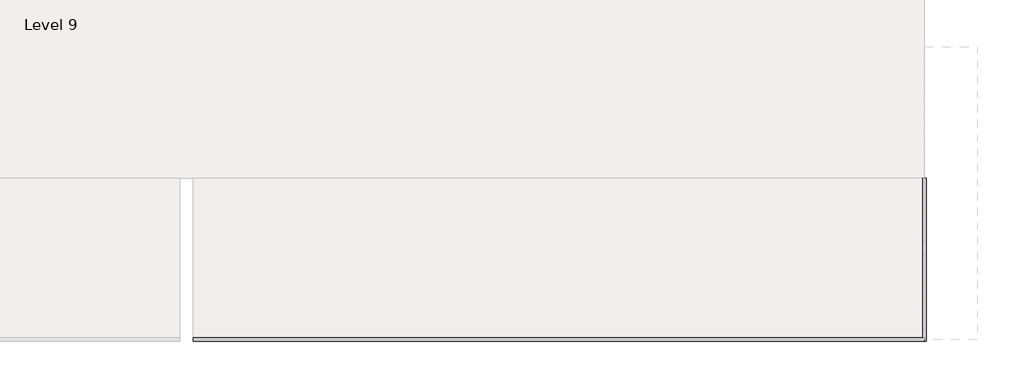
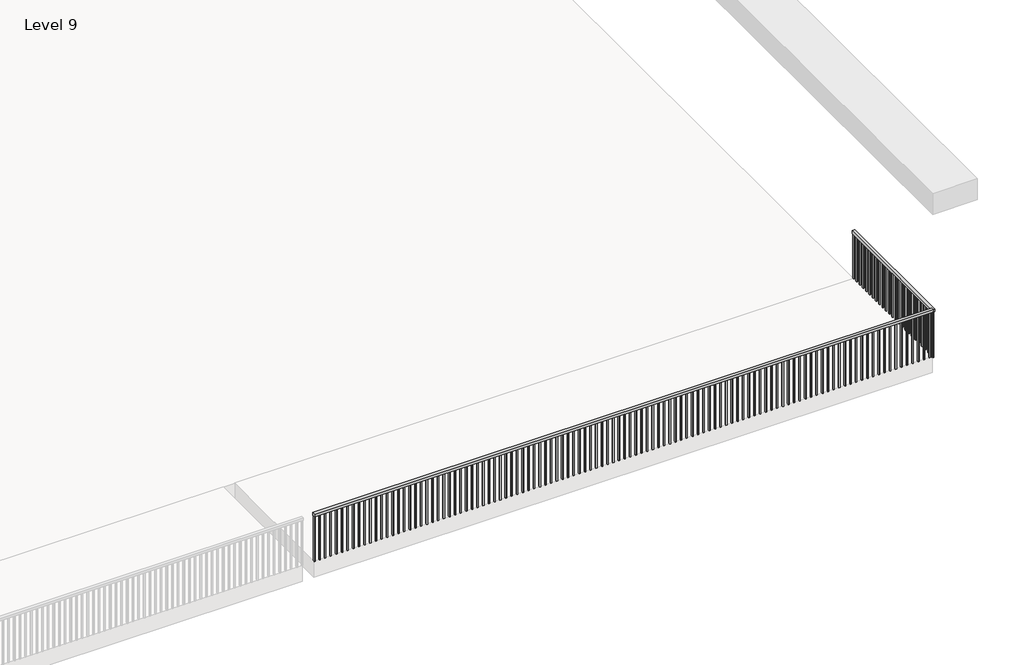
# One storey, part 2 of 5: 2 railings.
"""IFC4 building model written with IfcOpenShell, lengths in millimetres."""

from ifc_helpers import new_model, si_unit, frame, origin, place, context, project, spatial, polyline, outline, extrude, element, save

model = new_model("IFC4")

# Units and contexts
model_context = context("Model", 3, world=origin())
ifc_project = project(units=[si_unit("LENGTHUNIT", "METRE", prefix="MILLI")], contexts=[model_context])

# Site, building, storey
site = spatial("IfcSite", under=ifc_project)
building = spatial("IfcBuilding", under=site)
storey = spatial("IfcBuildingStorey", under=building, Name="Level 9", Elevation=9448.8)

# Railings
placement = place(None, origin())
element("IfcRailing", 1, ObjectType="Handrail - Rectangular", at=placement, inside=storey, context=model_context, shape_type="SweptSolid", body=[
    extrude(outline(polyline([(2981.3361222, -12911.7749501), (2981.3361222, -12860.9749501), (14106.5361222, -12860.9749501), (14106.5361222, -12911.7749501), (2981.3361222, -12911.7749501)])), frame((0.0, 0.0, 10312.4), z_axis=(0.0, 0.0, 1.0), x_axis=(1.0, 0.0, 0.0)), (0.0, 0.0, 1.0), 50.8),
    extrude(outline(polyline([(14046.2111222, -12895.8999501), (14046.2111222, -12876.8499501), (14065.2611222, -12876.8499501), (14065.2611222, -12895.8999501), (14046.2111222, -12895.8999501)])), frame((0.0, 0.0, 9448.8), z_axis=(0.0, 0.0, 1.0), x_axis=(1.0, 0.0, 0.0)), (0.0, 0.0, 1.0), 863.6),
    extrude(outline(polyline([(13944.6111222, -12895.8999501), (13944.6111222, -12876.8499501), (13963.6611222, -12876.8499501), (13963.6611222, -12895.8999501), (13944.6111222, -12895.8999501)])), frame((0.0, 0.0, 9448.8), z_axis=(0.0, 0.0, 1.0), x_axis=(1.0, 0.0, 0.0)), (0.0, 0.0, 1.0), 863.6),
    extrude(outline(polyline([(13843.0111222, -12895.8999501), (13843.0111222, -12876.8499501), (13862.0611222, -12876.8499501), (13862.0611222, -12895.8999501), (13843.0111222, -12895.8999501)])), frame((0.0, 0.0, 9448.8), z_axis=(0.0, 0.0, 1.0), x_axis=(1.0, 0.0, 0.0)), (0.0, 0.0, 1.0), 863.6),
    extrude(outline(polyline([(13741.4111222, -12895.8999501), (13741.4111222, -12876.8499501), (13760.4611222, -12876.8499501), (13760.4611222, -12895.8999501), (13741.4111222, -12895.8999501)])), frame((0.0, 0.0, 9448.8), z_axis=(0.0, 0.0, 1.0), x_axis=(1.0, 0.0, 0.0)), (0.0, 0.0, 1.0), 863.6),
    extrude(outline(polyline([(13639.8111222, -12895.8999501), (13639.8111222, -12876.8499501), (13658.8611222, -12876.8499501), (13658.8611222, -12895.8999501), (13639.8111222, -12895.8999501)])), frame((0.0, 0.0, 9448.8), z_axis=(0.0, 0.0, 1.0), x_axis=(1.0, 0.0, 0.0)), (0.0, 0.0, 1.0), 863.6),
    extrude(outline(polyline([(13538.2111222, -12895.8999501), (13538.2111222, -12876.8499501), (13557.2611222, -12876.8499501), (13557.2611222, -12895.8999501), (13538.2111222, -12895.8999501)])), frame((0.0, 0.0, 9448.8), z_axis=(0.0, 0.0, 1.0), x_axis=(1.0, 0.0, 0.0)), (0.0, 0.0, 1.0), 863.6),
    extrude(outline(polyline([(13436.6111222, -12895.8999501), (13436.6111222, -12876.8499501), (13455.6611222, -12876.8499501), (13455.6611222, -12895.8999501), (13436.6111222, -12895.8999501)])), frame((0.0, 0.0, 9448.8), z_axis=(0.0, 0.0, 1.0), x_axis=(1.0, 0.0, 0.0)), (0.0, 0.0, 1.0), 863.6),
    extrude(outline(polyline([(13335.0111222, -12895.8999501), (13335.0111222, -12876.8499501), (13354.0611222, -12876.8499501), (13354.0611222, -12895.8999501), (13335.0111222, -12895.8999501)])), frame((0.0, 0.0, 9448.8), z_axis=(0.0, 0.0, 1.0), x_axis=(1.0, 0.0, 0.0)), (0.0, 0.0, 1.0), 863.6),
    extrude(outline(polyline([(13233.4111222, -12895.8999501), (13233.4111222, -12876.8499501), (13252.4611222, -12876.8499501), (13252.4611222, -12895.8999501), (13233.4111222, -12895.8999501)])), frame((0.0, 0.0, 9448.8), z_axis=(0.0, 0.0, 1.0), x_axis=(1.0, 0.0, 0.0)), (0.0, 0.0, 1.0), 863.6),
    extrude(outline(polyline([(13131.8111222, -12895.8999501), (13131.8111222, -12876.8499501), (13150.8611222, -12876.8499501), (13150.8611222, -12895.8999501), (13131.8111222, -12895.8999501)])), frame((0.0, 0.0, 9448.8), z_axis=(0.0, 0.0, 1.0), x_axis=(1.0, 0.0, 0.0)), (0.0, 0.0, 1.0), 863.6),
    extrude(outline(polyline([(13030.2111222, -12895.8999501), (13030.2111222, -12876.8499501), (13049.2611222, -12876.8499501), (13049.2611222, -12895.8999501), (13030.2111222, -12895.8999501)])), frame((0.0, 0.0, 9448.8), z_axis=(0.0, 0.0, 1.0), x_axis=(1.0, 0.0, 0.0)), (0.0, 0.0, 1.0), 863.6),
    extrude(outline(polyline([(12928.6111222, -12895.8999501), (12928.6111222, -12876.8499501), (12947.6611222, -12876.8499501), (12947.6611222, -12895.8999501), (12928.6111222, -12895.8999501)])), frame((0.0, 0.0, 9448.8), z_axis=(0.0, 0.0, 1.0), x_axis=(1.0, 0.0, 0.0)), (0.0, 0.0, 1.0), 863.6),
    extrude(outline(polyline([(12827.0111222, -12895.8999501), (12827.0111222, -12876.8499501), (12846.0611222, -12876.8499501), (12846.0611222, -12895.8999501), (12827.0111222, -12895.8999501)])), frame((0.0, 0.0, 9448.8), z_axis=(0.0, 0.0, 1.0), x_axis=(1.0, 0.0, 0.0)), (0.0, 0.0, 1.0), 863.6),
    extrude(outline(polyline([(12725.4111222, -12895.8999501), (12725.4111222, -12876.8499501), (12744.4611222, -12876.8499501), (12744.4611222, -12895.8999501), (12725.4111222, -12895.8999501)])), frame((0.0, 0.0, 9448.8), z_axis=(0.0, 0.0, 1.0), x_axis=(1.0, 0.0, 0.0)), (0.0, 0.0, 1.0), 863.6),
    extrude(outline(polyline([(12623.8111222, -12895.8999501), (12623.8111222, -12876.8499501), (12642.8611222, -12876.8499501), (12642.8611222, -12895.8999501), (12623.8111222, -12895.8999501)])), frame((0.0, 0.0, 9448.8), z_axis=(0.0, 0.0, 1.0), x_axis=(1.0, 0.0, 0.0)), (0.0, 0.0, 1.0), 863.6),
    extrude(outline(polyline([(12522.2111222, -12895.8999501), (12522.2111222, -12876.8499501), (12541.2611222, -12876.8499501), (12541.2611222, -12895.8999501), (12522.2111222, -12895.8999501)])), frame((0.0, 0.0, 9448.8), z_axis=(0.0, 0.0, 1.0), x_axis=(1.0, 0.0, 0.0)), (0.0, 0.0, 1.0), 863.6),
    extrude(outline(polyline([(12420.6111222, -12895.8999501), (12420.6111222, -12876.8499501), (12439.6611222, -12876.8499501), (12439.6611222, -12895.8999501), (12420.6111222, -12895.8999501)])), frame((0.0, 0.0, 9448.8), z_axis=(0.0, 0.0, 1.0), x_axis=(1.0, 0.0, 0.0)), (0.0, 0.0, 1.0), 863.6),
    extrude(outline(polyline([(12319.0111222, -12895.8999501), (12319.0111222, -12876.8499501), (12338.0611222, -12876.8499501), (12338.0611222, -12895.8999501), (12319.0111222, -12895.8999501)])), frame((0.0, 0.0, 9448.8), z_axis=(0.0, 0.0, 1.0), x_axis=(1.0, 0.0, 0.0)), (0.0, 0.0, 1.0), 863.6),
    extrude(outline(polyline([(12217.4111222, -12895.8999501), (12217.4111222, -12876.8499501), (12236.4611222, -12876.8499501), (12236.4611222, -12895.8999501), (12217.4111222, -12895.8999501)])), frame((0.0, 0.0, 9448.8), z_axis=(0.0, 0.0, 1.0), x_axis=(1.0, 0.0, 0.0)), (0.0, 0.0, 1.0), 863.6),
    extrude(outline(polyline([(12115.8111222, -12895.8999501), (12115.8111222, -12876.8499501), (12134.8611222, -12876.8499501), (12134.8611222, -12895.8999501), (12115.8111222, -12895.8999501)])), frame((0.0, 0.0, 9448.8), z_axis=(0.0, 0.0, 1.0), x_axis=(1.0, 0.0, 0.0)), (0.0, 0.0, 1.0), 863.6),
    extrude(outline(polyline([(12014.2111222, -12895.8999501), (12014.2111222, -12876.8499501), (12033.2611222, -12876.8499501), (12033.2611222, -12895.8999501), (12014.2111222, -12895.8999501)])), frame((0.0, 0.0, 9448.8), z_axis=(0.0, 0.0, 1.0), x_axis=(1.0, 0.0, 0.0)), (0.0, 0.0, 1.0), 863.6),
    extrude(outline(polyline([(11912.6111222, -12895.8999501), (11912.6111222, -12876.8499501), (11931.6611222, -12876.8499501), (11931.6611222, -12895.8999501), (11912.6111222, -12895.8999501)])), frame((0.0, 0.0, 9448.8), z_axis=(0.0, 0.0, 1.0), x_axis=(1.0, 0.0, 0.0)), (0.0, 0.0, 1.0), 863.6),
    extrude(outline(polyline([(11811.0111222, -12895.8999501), (11811.0111222, -12876.8499501), (11830.0611222, -12876.8499501), (11830.0611222, -12895.8999501), (11811.0111222, -12895.8999501)])), frame((0.0, 0.0, 9448.8), z_axis=(0.0, 0.0, 1.0), x_axis=(1.0, 0.0, 0.0)), (0.0, 0.0, 1.0), 863.6),
    extrude(outline(polyline([(11709.4111222, -12895.8999501), (11709.4111222, -12876.8499501), (11728.4611222, -12876.8499501), (11728.4611222, -12895.8999501), (11709.4111222, -12895.8999501)])), frame((0.0, 0.0, 9448.8), z_axis=(0.0, 0.0, 1.0), x_axis=(1.0, 0.0, 0.0)), (0.0, 0.0, 1.0), 863.6),
    extrude(outline(polyline([(11607.8111222, -12895.8999501), (11607.8111222, -12876.8499501), (11626.8611222, -12876.8499501), (11626.8611222, -12895.8999501), (11607.8111222, -12895.8999501)])), frame((0.0, 0.0, 9448.8), z_axis=(0.0, 0.0, 1.0), x_axis=(1.0, 0.0, 0.0)), (0.0, 0.0, 1.0), 863.6),
    extrude(outline(polyline([(11506.2111222, -12895.8999501), (11506.2111222, -12876.8499501), (11525.2611222, -12876.8499501), (11525.2611222, -12895.8999501), (11506.2111222, -12895.8999501)])), frame((0.0, 0.0, 9448.8), z_axis=(0.0, 0.0, 1.0), x_axis=(1.0, 0.0, 0.0)), (0.0, 0.0, 1.0), 863.6),
    extrude(outline(polyline([(11404.6111222, -12895.8999501), (11404.6111222, -12876.8499501), (11423.6611222, -12876.8499501), (11423.6611222, -12895.8999501), (11404.6111222, -12895.8999501)])), frame((0.0, 0.0, 9448.8), z_axis=(0.0, 0.0, 1.0), x_axis=(1.0, 0.0, 0.0)), (0.0, 0.0, 1.0), 863.6),
    extrude(outline(polyline([(11303.0111222, -12895.8999501), (11303.0111222, -12876.8499501), (11322.0611222, -12876.8499501), (11322.0611222, -12895.8999501), (11303.0111222, -12895.8999501)])), frame((0.0, 0.0, 9448.8), z_axis=(0.0, 0.0, 1.0), x_axis=(1.0, 0.0, 0.0)), (0.0, 0.0, 1.0), 863.6),
    extrude(outline(polyline([(11201.4111222, -12895.8999501), (11201.4111222, -12876.8499501), (11220.4611222, -12876.8499501), (11220.4611222, -12895.8999501), (11201.4111222, -12895.8999501)])), frame((0.0, 0.0, 9448.8), z_axis=(0.0, 0.0, 1.0), x_axis=(1.0, 0.0, 0.0)), (0.0, 0.0, 1.0), 863.6),
    extrude(outline(polyline([(11099.8111222, -12895.8999501), (11099.8111222, -12876.8499501), (11118.8611222, -12876.8499501), (11118.8611222, -12895.8999501), (11099.8111222, -12895.8999501)])), frame((0.0, 0.0, 9448.8), z_axis=(0.0, 0.0, 1.0), x_axis=(1.0, 0.0, 0.0)), (0.0, 0.0, 1.0), 863.6),
    extrude(outline(polyline([(10998.2111222, -12895.8999501), (10998.2111222, -12876.8499501), (11017.2611222, -12876.8499501), (11017.2611222, -12895.8999501), (10998.2111222, -12895.8999501)])), frame((0.0, 0.0, 9448.8), z_axis=(0.0, 0.0, 1.0), x_axis=(1.0, 0.0, 0.0)), (0.0, 0.0, 1.0), 863.6),
    extrude(outline(polyline([(10896.6111222, -12895.8999501), (10896.6111222, -12876.8499501), (10915.6611222, -12876.8499501), (10915.6611222, -12895.8999501), (10896.6111222, -12895.8999501)])), frame((0.0, 0.0, 9448.8), z_axis=(0.0, 0.0, 1.0), x_axis=(1.0, 0.0, 0.0)), (0.0, 0.0, 1.0), 863.6),
    extrude(outline(polyline([(10795.0111222, -12895.8999501), (10795.0111222, -12876.8499501), (10814.0611222, -12876.8499501), (10814.0611222, -12895.8999501), (10795.0111222, -12895.8999501)])), frame((0.0, 0.0, 9448.8), z_axis=(0.0, 0.0, 1.0), x_axis=(1.0, 0.0, 0.0)), (0.0, 0.0, 1.0), 863.6),
    extrude(outline(polyline([(10693.4111222, -12895.8999501), (10693.4111222, -12876.8499501), (10712.4611222, -12876.8499501), (10712.4611222, -12895.8999501), (10693.4111222, -12895.8999501)])), frame((0.0, 0.0, 9448.8), z_axis=(0.0, 0.0, 1.0), x_axis=(1.0, 0.0, 0.0)), (0.0, 0.0, 1.0), 863.6),
    extrude(outline(polyline([(10591.8111222, -12895.8999501), (10591.8111222, -12876.8499501), (10610.8611222, -12876.8499501), (10610.8611222, -12895.8999501), (10591.8111222, -12895.8999501)])), frame((0.0, 0.0, 9448.8), z_axis=(0.0, 0.0, 1.0), x_axis=(1.0, 0.0, 0.0)), (0.0, 0.0, 1.0), 863.6),
    extrude(outline(polyline([(10490.2111222, -12895.8999501), (10490.2111222, -12876.8499501), (10509.2611222, -12876.8499501), (10509.2611222, -12895.8999501), (10490.2111222, -12895.8999501)])), frame((0.0, 0.0, 9448.8), z_axis=(0.0, 0.0, 1.0), x_axis=(1.0, 0.0, 0.0)), (0.0, 0.0, 1.0), 863.6),
    extrude(outline(polyline([(10388.6111222, -12895.8999501), (10388.6111222, -12876.8499501), (10407.6611222, -12876.8499501), (10407.6611222, -12895.8999501), (10388.6111222, -12895.8999501)])), frame((0.0, 0.0, 9448.8), z_axis=(0.0, 0.0, 1.0), x_axis=(1.0, 0.0, 0.0)), (0.0, 0.0, 1.0), 863.6),
    extrude(outline(polyline([(10287.0111222, -12895.8999501), (10287.0111222, -12876.8499501), (10306.0611222, -12876.8499501), (10306.0611222, -12895.8999501), (10287.0111222, -12895.8999501)])), frame((0.0, 0.0, 9448.8), z_axis=(0.0, 0.0, 1.0), x_axis=(1.0, 0.0, 0.0)), (0.0, 0.0, 1.0), 863.6),
    extrude(outline(polyline([(10185.4111222, -12895.8999501), (10185.4111222, -12876.8499501), (10204.4611222, -12876.8499501), (10204.4611222, -12895.8999501), (10185.4111222, -12895.8999501)])), frame((0.0, 0.0, 9448.8), z_axis=(0.0, 0.0, 1.0), x_axis=(1.0, 0.0, 0.0)), (0.0, 0.0, 1.0), 863.6),
    extrude(outline(polyline([(10083.8111222, -12895.8999501), (10083.8111222, -12876.8499501), (10102.8611222, -12876.8499501), (10102.8611222, -12895.8999501), (10083.8111222, -12895.8999501)])), frame((0.0, 0.0, 9448.8), z_axis=(0.0, 0.0, 1.0), x_axis=(1.0, 0.0, 0.0)), (0.0, 0.0, 1.0), 863.6),
    extrude(outline(polyline([(9982.2111222, -12895.8999501), (9982.2111222, -12876.8499501), (10001.2611222, -12876.8499501), (10001.2611222, -12895.8999501), (9982.2111222, -12895.8999501)])), frame((0.0, 0.0, 9448.8), z_axis=(0.0, 0.0, 1.0), x_axis=(1.0, 0.0, 0.0)), (0.0, 0.0, 1.0), 863.6),
    extrude(outline(polyline([(9880.6111222, -12895.8999501), (9880.6111222, -12876.8499501), (9899.6611222, -12876.8499501), (9899.6611222, -12895.8999501), (9880.6111222, -12895.8999501)])), frame((0.0, 0.0, 9448.8), z_axis=(0.0, 0.0, 1.0), x_axis=(1.0, 0.0, 0.0)), (0.0, 0.0, 1.0), 863.6),
    extrude(outline(polyline([(9779.0111222, -12895.8999501), (9779.0111222, -12876.8499501), (9798.0611222, -12876.8499501), (9798.0611222, -12895.8999501), (9779.0111222, -12895.8999501)])), frame((0.0, 0.0, 9448.8), z_axis=(0.0, 0.0, 1.0), x_axis=(1.0, 0.0, 0.0)), (0.0, 0.0, 1.0), 863.6),
    extrude(outline(polyline([(9677.4111222, -12895.8999501), (9677.4111222, -12876.8499501), (9696.4611222, -12876.8499501), (9696.4611222, -12895.8999501), (9677.4111222, -12895.8999501)])), frame((0.0, 0.0, 9448.8), z_axis=(0.0, 0.0, 1.0), x_axis=(1.0, 0.0, 0.0)), (0.0, 0.0, 1.0), 863.6),
    extrude(outline(polyline([(9575.8111222, -12895.8999501), (9575.8111222, -12876.8499501), (9594.8611222, -12876.8499501), (9594.8611222, -12895.8999501), (9575.8111222, -12895.8999501)])), frame((0.0, 0.0, 9448.8), z_axis=(0.0, 0.0, 1.0), x_axis=(1.0, 0.0, 0.0)), (0.0, 0.0, 1.0), 863.6),
    extrude(outline(polyline([(9474.2111222, -12895.8999501), (9474.2111222, -12876.8499501), (9493.2611222, -12876.8499501), (9493.2611222, -12895.8999501), (9474.2111222, -12895.8999501)])), frame((0.0, 0.0, 9448.8), z_axis=(0.0, 0.0, 1.0), x_axis=(1.0, 0.0, 0.0)), (0.0, 0.0, 1.0), 863.6),
    extrude(outline(polyline([(9372.6111222, -12895.8999501), (9372.6111222, -12876.8499501), (9391.6611222, -12876.8499501), (9391.6611222, -12895.8999501), (9372.6111222, -12895.8999501)])), frame((0.0, 0.0, 9448.8), z_axis=(0.0, 0.0, 1.0), x_axis=(1.0, 0.0, 0.0)), (0.0, 0.0, 1.0), 863.6),
    extrude(outline(polyline([(9271.0111222, -12895.8999501), (9271.0111222, -12876.8499501), (9290.0611222, -12876.8499501), (9290.0611222, -12895.8999501), (9271.0111222, -12895.8999501)])), frame((0.0, 0.0, 9448.8), z_axis=(0.0, 0.0, 1.0), x_axis=(1.0, 0.0, 0.0)), (0.0, 0.0, 1.0), 863.6),
    extrude(outline(polyline([(9169.4111222, -12895.8999501), (9169.4111222, -12876.8499501), (9188.4611222, -12876.8499501), (9188.4611222, -12895.8999501), (9169.4111222, -12895.8999501)])), frame((0.0, 0.0, 9448.8), z_axis=(0.0, 0.0, 1.0), x_axis=(1.0, 0.0, 0.0)), (0.0, 0.0, 1.0), 863.6),
    extrude(outline(polyline([(9067.8111222, -12895.8999501), (9067.8111222, -12876.8499501), (9086.8611222, -12876.8499501), (9086.8611222, -12895.8999501), (9067.8111222, -12895.8999501)])), frame((0.0, 0.0, 9448.8), z_axis=(0.0, 0.0, 1.0), x_axis=(1.0, 0.0, 0.0)), (0.0, 0.0, 1.0), 863.6),
    extrude(outline(polyline([(8966.2111222, -12895.8999501), (8966.2111222, -12876.8499501), (8985.2611222, -12876.8499501), (8985.2611222, -12895.8999501), (8966.2111222, -12895.8999501)])), frame((0.0, 0.0, 9448.8), z_axis=(0.0, 0.0, 1.0), x_axis=(1.0, 0.0, 0.0)), (0.0, 0.0, 1.0), 863.6),
    extrude(outline(polyline([(8864.6111222, -12895.8999501), (8864.6111222, -12876.8499501), (8883.6611222, -12876.8499501), (8883.6611222, -12895.8999501), (8864.6111222, -12895.8999501)])), frame((0.0, 0.0, 9448.8), z_axis=(0.0, 0.0, 1.0), x_axis=(1.0, 0.0, 0.0)), (0.0, 0.0, 1.0), 863.6),
    extrude(outline(polyline([(8763.0111222, -12895.8999501), (8763.0111222, -12876.8499501), (8782.0611222, -12876.8499501), (8782.0611222, -12895.8999501), (8763.0111222, -12895.8999501)])), frame((0.0, 0.0, 9448.8), z_axis=(0.0, 0.0, 1.0), x_axis=(1.0, 0.0, 0.0)), (0.0, 0.0, 1.0), 863.6),
    extrude(outline(polyline([(8661.4111222, -12895.8999501), (8661.4111222, -12876.8499501), (8680.4611222, -12876.8499501), (8680.4611222, -12895.8999501), (8661.4111222, -12895.8999501)])), frame((0.0, 0.0, 9448.8), z_axis=(0.0, 0.0, 1.0), x_axis=(1.0, 0.0, 0.0)), (0.0, 0.0, 1.0), 863.6),
    extrude(outline(polyline([(8559.8111222, -12895.8999501), (8559.8111222, -12876.8499501), (8578.8611222, -12876.8499501), (8578.8611222, -12895.8999501), (8559.8111222, -12895.8999501)])), frame((0.0, 0.0, 9448.8), z_axis=(0.0, 0.0, 1.0), x_axis=(1.0, 0.0, 0.0)), (0.0, 0.0, 1.0), 863.6),
    extrude(outline(polyline([(8458.2111222, -12895.8999501), (8458.2111222, -12876.8499501), (8477.2611222, -12876.8499501), (8477.2611222, -12895.8999501), (8458.2111222, -12895.8999501)])), frame((0.0, 0.0, 9448.8), z_axis=(0.0, 0.0, 1.0), x_axis=(1.0, 0.0, 0.0)), (0.0, 0.0, 1.0), 863.6),
    extrude(outline(polyline([(8356.6111222, -12895.8999501), (8356.6111222, -12876.8499501), (8375.6611222, -12876.8499501), (8375.6611222, -12895.8999501), (8356.6111222, -12895.8999501)])), frame((0.0, 0.0, 9448.8), z_axis=(0.0, 0.0, 1.0), x_axis=(1.0, 0.0, 0.0)), (0.0, 0.0, 1.0), 863.6),
    extrude(outline(polyline([(8255.0111222, -12895.8999501), (8255.0111222, -12876.8499501), (8274.0611222, -12876.8499501), (8274.0611222, -12895.8999501), (8255.0111222, -12895.8999501)])), frame((0.0, 0.0, 9448.8), z_axis=(0.0, 0.0, 1.0), x_axis=(1.0, 0.0, 0.0)), (0.0, 0.0, 1.0), 863.6),
    extrude(outline(polyline([(8153.4111222, -12895.8999501), (8153.4111222, -12876.8499501), (8172.4611222, -12876.8499501), (8172.4611222, -12895.8999501), (8153.4111222, -12895.8999501)])), frame((0.0, 0.0, 9448.8), z_axis=(0.0, 0.0, 1.0), x_axis=(1.0, 0.0, 0.0)), (0.0, 0.0, 1.0), 863.6),
    extrude(outline(polyline([(8051.8111222, -12895.8999501), (8051.8111222, -12876.8499501), (8070.8611222, -12876.8499501), (8070.8611222, -12895.8999501), (8051.8111222, -12895.8999501)])), frame((0.0, 0.0, 9448.8), z_axis=(0.0, 0.0, 1.0), x_axis=(1.0, 0.0, 0.0)), (0.0, 0.0, 1.0), 863.6),
    extrude(outline(polyline([(7950.2111222, -12895.8999501), (7950.2111222, -12876.8499501), (7969.2611222, -12876.8499501), (7969.2611222, -12895.8999501), (7950.2111222, -12895.8999501)])), frame((0.0, 0.0, 9448.8), z_axis=(0.0, 0.0, 1.0), x_axis=(1.0, 0.0, 0.0)), (0.0, 0.0, 1.0), 863.6),
    extrude(outline(polyline([(7848.6111222, -12895.8999501), (7848.6111222, -12876.8499501), (7867.6611222, -12876.8499501), (7867.6611222, -12895.8999501), (7848.6111222, -12895.8999501)])), frame((0.0, 0.0, 9448.8), z_axis=(0.0, 0.0, 1.0), x_axis=(1.0, 0.0, 0.0)), (0.0, 0.0, 1.0), 863.6),
    extrude(outline(polyline([(7747.0111222, -12895.8999501), (7747.0111222, -12876.8499501), (7766.0611222, -12876.8499501), (7766.0611222, -12895.8999501), (7747.0111222, -12895.8999501)])), frame((0.0, 0.0, 9448.8), z_axis=(0.0, 0.0, 1.0), x_axis=(1.0, 0.0, 0.0)), (0.0, 0.0, 1.0), 863.6),
    extrude(outline(polyline([(7645.4111222, -12895.8999501), (7645.4111222, -12876.8499501), (7664.4611222, -12876.8499501), (7664.4611222, -12895.8999501), (7645.4111222, -12895.8999501)])), frame((0.0, 0.0, 9448.8), z_axis=(0.0, 0.0, 1.0), x_axis=(1.0, 0.0, 0.0)), (0.0, 0.0, 1.0), 863.6),
    extrude(outline(polyline([(7543.8111222, -12895.8999501), (7543.8111222, -12876.8499501), (7562.8611222, -12876.8499501), (7562.8611222, -12895.8999501), (7543.8111222, -12895.8999501)])), frame((0.0, 0.0, 9448.8), z_axis=(0.0, 0.0, 1.0), x_axis=(1.0, 0.0, 0.0)), (0.0, 0.0, 1.0), 863.6),
    extrude(outline(polyline([(7442.2111222, -12895.8999501), (7442.2111222, -12876.8499501), (7461.2611222, -12876.8499501), (7461.2611222, -12895.8999501), (7442.2111222, -12895.8999501)])), frame((0.0, 0.0, 9448.8), z_axis=(0.0, 0.0, 1.0), x_axis=(1.0, 0.0, 0.0)), (0.0, 0.0, 1.0), 863.6),
    extrude(outline(polyline([(7340.6111222, -12895.8999501), (7340.6111222, -12876.8499501), (7359.6611222, -12876.8499501), (7359.6611222, -12895.8999501), (7340.6111222, -12895.8999501)])), frame((0.0, 0.0, 9448.8), z_axis=(0.0, 0.0, 1.0), x_axis=(1.0, 0.0, 0.0)), (0.0, 0.0, 1.0), 863.6),
    extrude(outline(polyline([(7239.0111222, -12895.8999501), (7239.0111222, -12876.8499501), (7258.0611222, -12876.8499501), (7258.0611222, -12895.8999501), (7239.0111222, -12895.8999501)])), frame((0.0, 0.0, 9448.8), z_axis=(0.0, 0.0, 1.0), x_axis=(1.0, 0.0, 0.0)), (0.0, 0.0, 1.0), 863.6),
    extrude(outline(polyline([(7137.4111222, -12895.8999501), (7137.4111222, -12876.8499501), (7156.4611222, -12876.8499501), (7156.4611222, -12895.8999501), (7137.4111222, -12895.8999501)])), frame((0.0, 0.0, 9448.8), z_axis=(0.0, 0.0, 1.0), x_axis=(1.0, 0.0, 0.0)), (0.0, 0.0, 1.0), 863.6),
    extrude(outline(polyline([(7035.8111222, -12895.8999501), (7035.8111222, -12876.8499501), (7054.8611222, -12876.8499501), (7054.8611222, -12895.8999501), (7035.8111222, -12895.8999501)])), frame((0.0, 0.0, 9448.8), z_axis=(0.0, 0.0, 1.0), x_axis=(1.0, 0.0, 0.0)), (0.0, 0.0, 1.0), 863.6),
    extrude(outline(polyline([(6934.2111222, -12895.8999501), (6934.2111222, -12876.8499501), (6953.2611222, -12876.8499501), (6953.2611222, -12895.8999501), (6934.2111222, -12895.8999501)])), frame((0.0, 0.0, 9448.8), z_axis=(0.0, 0.0, 1.0), x_axis=(1.0, 0.0, 0.0)), (0.0, 0.0, 1.0), 863.6),
    extrude(outline(polyline([(6832.6111222, -12895.8999501), (6832.6111222, -12876.8499501), (6851.6611222, -12876.8499501), (6851.6611222, -12895.8999501), (6832.6111222, -12895.8999501)])), frame((0.0, 0.0, 9448.8), z_axis=(0.0, 0.0, 1.0), x_axis=(1.0, 0.0, 0.0)), (0.0, 0.0, 1.0), 863.6),
    extrude(outline(polyline([(6731.0111222, -12895.8999501), (6731.0111222, -12876.8499501), (6750.0611222, -12876.8499501), (6750.0611222, -12895.8999501), (6731.0111222, -12895.8999501)])), frame((0.0, 0.0, 9448.8), z_axis=(0.0, 0.0, 1.0), x_axis=(1.0, 0.0, 0.0)), (0.0, 0.0, 1.0), 863.6),
    extrude(outline(polyline([(6629.4111222, -12895.8999501), (6629.4111222, -12876.8499501), (6648.4611222, -12876.8499501), (6648.4611222, -12895.8999501), (6629.4111222, -12895.8999501)])), frame((0.0, 0.0, 9448.8), z_axis=(0.0, 0.0, 1.0), x_axis=(1.0, 0.0, 0.0)), (0.0, 0.0, 1.0), 863.6),
    extrude(outline(polyline([(6527.8111222, -12895.8999501), (6527.8111222, -12876.8499501), (6546.8611222, -12876.8499501), (6546.8611222, -12895.8999501), (6527.8111222, -12895.8999501)])), frame((0.0, 0.0, 9448.8), z_axis=(0.0, 0.0, 1.0), x_axis=(1.0, 0.0, 0.0)), (0.0, 0.0, 1.0), 863.6),
    extrude(outline(polyline([(6426.2111222, -12895.8999501), (6426.2111222, -12876.8499501), (6445.2611222, -12876.8499501), (6445.2611222, -12895.8999501), (6426.2111222, -12895.8999501)])), frame((0.0, 0.0, 9448.8), z_axis=(0.0, 0.0, 1.0), x_axis=(1.0, 0.0, 0.0)), (0.0, 0.0, 1.0), 863.6),
    extrude(outline(polyline([(6324.6111222, -12895.8999501), (6324.6111222, -12876.8499501), (6343.6611222, -12876.8499501), (6343.6611222, -12895.8999501), (6324.6111222, -12895.8999501)])), frame((0.0, 0.0, 9448.8), z_axis=(0.0, 0.0, 1.0), x_axis=(1.0, 0.0, 0.0)), (0.0, 0.0, 1.0), 863.6),
    extrude(outline(polyline([(6223.0111222, -12895.8999501), (6223.0111222, -12876.8499501), (6242.0611222, -12876.8499501), (6242.0611222, -12895.8999501), (6223.0111222, -12895.8999501)])), frame((0.0, 0.0, 9448.8), z_axis=(0.0, 0.0, 1.0), x_axis=(1.0, 0.0, 0.0)), (0.0, 0.0, 1.0), 863.6),
    extrude(outline(polyline([(6121.4111222, -12895.8999501), (6121.4111222, -12876.8499501), (6140.4611222, -12876.8499501), (6140.4611222, -12895.8999501), (6121.4111222, -12895.8999501)])), frame((0.0, 0.0, 9448.8), z_axis=(0.0, 0.0, 1.0), x_axis=(1.0, 0.0, 0.0)), (0.0, 0.0, 1.0), 863.6),
    extrude(outline(polyline([(6019.8111222, -12895.8999501), (6019.8111222, -12876.8499501), (6038.8611222, -12876.8499501), (6038.8611222, -12895.8999501), (6019.8111222, -12895.8999501)])), frame((0.0, 0.0, 9448.8), z_axis=(0.0, 0.0, 1.0), x_axis=(1.0, 0.0, 0.0)), (0.0, 0.0, 1.0), 863.6),
    extrude(outline(polyline([(5918.2111222, -12895.8999501), (5918.2111222, -12876.8499501), (5937.2611222, -12876.8499501), (5937.2611222, -12895.8999501), (5918.2111222, -12895.8999501)])), frame((0.0, 0.0, 9448.8), z_axis=(0.0, 0.0, 1.0), x_axis=(1.0, 0.0, 0.0)), (0.0, 0.0, 1.0), 863.6),
    extrude(outline(polyline([(5816.6111222, -12895.8999501), (5816.6111222, -12876.8499501), (5835.6611222, -12876.8499501), (5835.6611222, -12895.8999501), (5816.6111222, -12895.8999501)])), frame((0.0, 0.0, 9448.8), z_axis=(0.0, 0.0, 1.0), x_axis=(1.0, 0.0, 0.0)), (0.0, 0.0, 1.0), 863.6),
    extrude(outline(polyline([(5715.0111222, -12895.8999501), (5715.0111222, -12876.8499501), (5734.0611222, -12876.8499501), (5734.0611222, -12895.8999501), (5715.0111222, -12895.8999501)])), frame((0.0, 0.0, 9448.8), z_axis=(0.0, 0.0, 1.0), x_axis=(1.0, 0.0, 0.0)), (0.0, 0.0, 1.0), 863.6),
    extrude(outline(polyline([(5613.4111222, -12895.8999501), (5613.4111222, -12876.8499501), (5632.4611222, -12876.8499501), (5632.4611222, -12895.8999501), (5613.4111222, -12895.8999501)])), frame((0.0, 0.0, 9448.8), z_axis=(0.0, 0.0, 1.0), x_axis=(1.0, 0.0, 0.0)), (0.0, 0.0, 1.0), 863.6),
    extrude(outline(polyline([(5511.8111222, -12895.8999501), (5511.8111222, -12876.8499501), (5530.8611222, -12876.8499501), (5530.8611222, -12895.8999501), (5511.8111222, -12895.8999501)])), frame((0.0, 0.0, 9448.8), z_axis=(0.0, 0.0, 1.0), x_axis=(1.0, 0.0, 0.0)), (0.0, 0.0, 1.0), 863.6),
    extrude(outline(polyline([(5410.2111222, -12895.8999501), (5410.2111222, -12876.8499501), (5429.2611222, -12876.8499501), (5429.2611222, -12895.8999501), (5410.2111222, -12895.8999501)])), frame((0.0, 0.0, 9448.8), z_axis=(0.0, 0.0, 1.0), x_axis=(1.0, 0.0, 0.0)), (0.0, 0.0, 1.0), 863.6),
    extrude(outline(polyline([(5308.6111222, -12895.8999501), (5308.6111222, -12876.8499501), (5327.6611222, -12876.8499501), (5327.6611222, -12895.8999501), (5308.6111222, -12895.8999501)])), frame((0.0, 0.0, 9448.8), z_axis=(0.0, 0.0, 1.0), x_axis=(1.0, 0.0, 0.0)), (0.0, 0.0, 1.0), 863.6),
    extrude(outline(polyline([(5207.0111222, -12895.8999501), (5207.0111222, -12876.8499501), (5226.0611222, -12876.8499501), (5226.0611222, -12895.8999501), (5207.0111222, -12895.8999501)])), frame((0.0, 0.0, 9448.8), z_axis=(0.0, 0.0, 1.0), x_axis=(1.0, 0.0, 0.0)), (0.0, 0.0, 1.0), 863.6),
    extrude(outline(polyline([(5105.4111222, -12895.8999501), (5105.4111222, -12876.8499501), (5124.4611222, -12876.8499501), (5124.4611222, -12895.8999501), (5105.4111222, -12895.8999501)])), frame((0.0, 0.0, 9448.8), z_axis=(0.0, 0.0, 1.0), x_axis=(1.0, 0.0, 0.0)), (0.0, 0.0, 1.0), 863.6),
    extrude(outline(polyline([(5003.8111222, -12895.8999501), (5003.8111222, -12876.8499501), (5022.8611222, -12876.8499501), (5022.8611222, -12895.8999501), (5003.8111222, -12895.8999501)])), frame((0.0, 0.0, 9448.8), z_axis=(0.0, 0.0, 1.0), x_axis=(1.0, 0.0, 0.0)), (0.0, 0.0, 1.0), 863.6),
    extrude(outline(polyline([(4902.2111222, -12895.8999501), (4902.2111222, -12876.8499501), (4921.2611222, -12876.8499501), (4921.2611222, -12895.8999501), (4902.2111222, -12895.8999501)])), frame((0.0, 0.0, 9448.8), z_axis=(0.0, 0.0, 1.0), x_axis=(1.0, 0.0, 0.0)), (0.0, 0.0, 1.0), 863.6),
    extrude(outline(polyline([(4800.6111222, -12895.8999501), (4800.6111222, -12876.8499501), (4819.6611222, -12876.8499501), (4819.6611222, -12895.8999501), (4800.6111222, -12895.8999501)])), frame((0.0, 0.0, 9448.8), z_axis=(0.0, 0.0, 1.0), x_axis=(1.0, 0.0, 0.0)), (0.0, 0.0, 1.0), 863.6),
    extrude(outline(polyline([(4699.0111222, -12895.8999501), (4699.0111222, -12876.8499501), (4718.0611222, -12876.8499501), (4718.0611222, -12895.8999501), (4699.0111222, -12895.8999501)])), frame((0.0, 0.0, 9448.8), z_axis=(0.0, 0.0, 1.0), x_axis=(1.0, 0.0, 0.0)), (0.0, 0.0, 1.0), 863.6),
    extrude(outline(polyline([(4597.4111222, -12895.8999501), (4597.4111222, -12876.8499501), (4616.4611222, -12876.8499501), (4616.4611222, -12895.8999501), (4597.4111222, -12895.8999501)])), frame((0.0, 0.0, 9448.8), z_axis=(0.0, 0.0, 1.0), x_axis=(1.0, 0.0, 0.0)), (0.0, 0.0, 1.0), 863.6),
    extrude(outline(polyline([(4495.8111222, -12895.8999501), (4495.8111222, -12876.8499501), (4514.8611222, -12876.8499501), (4514.8611222, -12895.8999501), (4495.8111222, -12895.8999501)])), frame((0.0, 0.0, 9448.8), z_axis=(0.0, 0.0, 1.0), x_axis=(1.0, 0.0, 0.0)), (0.0, 0.0, 1.0), 863.6),
    extrude(outline(polyline([(4394.2111222, -12895.8999501), (4394.2111222, -12876.8499501), (4413.2611222, -12876.8499501), (4413.2611222, -12895.8999501), (4394.2111222, -12895.8999501)])), frame((0.0, 0.0, 9448.8), z_axis=(0.0, 0.0, 1.0), x_axis=(1.0, 0.0, 0.0)), (0.0, 0.0, 1.0), 863.6),
    extrude(outline(polyline([(4292.6111222, -12895.8999501), (4292.6111222, -12876.8499501), (4311.6611222, -12876.8499501), (4311.6611222, -12895.8999501), (4292.6111222, -12895.8999501)])), frame((0.0, 0.0, 9448.8), z_axis=(0.0, 0.0, 1.0), x_axis=(1.0, 0.0, 0.0)), (0.0, 0.0, 1.0), 863.6),
    extrude(outline(polyline([(4191.0111222, -12895.8999501), (4191.0111222, -12876.8499501), (4210.0611222, -12876.8499501), (4210.0611222, -12895.8999501), (4191.0111222, -12895.8999501)])), frame((0.0, 0.0, 9448.8), z_axis=(0.0, 0.0, 1.0), x_axis=(1.0, 0.0, 0.0)), (0.0, 0.0, 1.0), 863.6),
    extrude(outline(polyline([(4089.4111222, -12895.8999501), (4089.4111222, -12876.8499501), (4108.4611222, -12876.8499501), (4108.4611222, -12895.8999501), (4089.4111222, -12895.8999501)])), frame((0.0, 0.0, 9448.8), z_axis=(0.0, 0.0, 1.0), x_axis=(1.0, 0.0, 0.0)), (0.0, 0.0, 1.0), 863.6),
    extrude(outline(polyline([(3987.8111222, -12895.8999501), (3987.8111222, -12876.8499501), (4006.8611222, -12876.8499501), (4006.8611222, -12895.8999501), (3987.8111222, -12895.8999501)])), frame((0.0, 0.0, 9448.8), z_axis=(0.0, 0.0, 1.0), x_axis=(1.0, 0.0, 0.0)), (0.0, 0.0, 1.0), 863.6),
    extrude(outline(polyline([(3886.2111222, -12895.8999501), (3886.2111222, -12876.8499501), (3905.2611222, -12876.8499501), (3905.2611222, -12895.8999501), (3886.2111222, -12895.8999501)])), frame((0.0, 0.0, 9448.8), z_axis=(0.0, 0.0, 1.0), x_axis=(1.0, 0.0, 0.0)), (0.0, 0.0, 1.0), 863.6),
    extrude(outline(polyline([(3784.6111222, -12895.8999501), (3784.6111222, -12876.8499501), (3803.6611222, -12876.8499501), (3803.6611222, -12895.8999501), (3784.6111222, -12895.8999501)])), frame((0.0, 0.0, 9448.8), z_axis=(0.0, 0.0, 1.0), x_axis=(1.0, 0.0, 0.0)), (0.0, 0.0, 1.0), 863.6),
    extrude(outline(polyline([(3683.0111222, -12895.8999501), (3683.0111222, -12876.8499501), (3702.0611222, -12876.8499501), (3702.0611222, -12895.8999501), (3683.0111222, -12895.8999501)])), frame((0.0, 0.0, 9448.8), z_axis=(0.0, 0.0, 1.0), x_axis=(1.0, 0.0, 0.0)), (0.0, 0.0, 1.0), 863.6),
    extrude(outline(polyline([(3581.4111222, -12895.8999501), (3581.4111222, -12876.8499501), (3600.4611222, -12876.8499501), (3600.4611222, -12895.8999501), (3581.4111222, -12895.8999501)])), frame((0.0, 0.0, 9448.8), z_axis=(0.0, 0.0, 1.0), x_axis=(1.0, 0.0, 0.0)), (0.0, 0.0, 1.0), 863.6),
    extrude(outline(polyline([(3479.8111222, -12895.8999501), (3479.8111222, -12876.8499501), (3498.8611222, -12876.8499501), (3498.8611222, -12895.8999501), (3479.8111222, -12895.8999501)])), frame((0.0, 0.0, 9448.8), z_axis=(0.0, 0.0, 1.0), x_axis=(1.0, 0.0, 0.0)), (0.0, 0.0, 1.0), 863.6),
    extrude(outline(polyline([(3378.2111222, -12895.8999501), (3378.2111222, -12876.8499501), (3397.2611222, -12876.8499501), (3397.2611222, -12895.8999501), (3378.2111222, -12895.8999501)])), frame((0.0, 0.0, 9448.8), z_axis=(0.0, 0.0, 1.0), x_axis=(1.0, 0.0, 0.0)), (0.0, 0.0, 1.0), 863.6),
    extrude(outline(polyline([(3276.6111222, -12895.8999501), (3276.6111222, -12876.8499501), (3295.6611222, -12876.8499501), (3295.6611222, -12895.8999501), (3276.6111222, -12895.8999501)])), frame((0.0, 0.0, 9448.8), z_axis=(0.0, 0.0, 1.0), x_axis=(1.0, 0.0, 0.0)), (0.0, 0.0, 1.0), 863.6),
    extrude(outline(polyline([(3175.0111222, -12895.8999501), (3175.0111222, -12876.8499501), (3194.0611222, -12876.8499501), (3194.0611222, -12895.8999501), (3175.0111222, -12895.8999501)])), frame((0.0, 0.0, 9448.8), z_axis=(0.0, 0.0, 1.0), x_axis=(1.0, 0.0, 0.0)), (0.0, 0.0, 1.0), 863.6),
    extrude(outline(polyline([(3073.4111222, -12895.8999501), (3073.4111222, -12876.8499501), (3092.4611222, -12876.8499501), (3092.4611222, -12895.8999501), (3073.4111222, -12895.8999501)])), frame((0.0, 0.0, 9448.8), z_axis=(0.0, 0.0, 1.0), x_axis=(1.0, 0.0, 0.0)), (0.0, 0.0, 1.0), 863.6),
    extrude(outline(polyline([(14087.4861222, -12895.8999501), (14087.4861222, -12876.8499501), (14106.5361222, -12876.8499501), (14106.5361222, -12895.8999501), (14087.4861222, -12895.8999501)])), frame((0.0, 0.0, 9448.8), z_axis=(0.0, 0.0, 1.0), x_axis=(1.0, 0.0, 0.0)), (0.0, 0.0, 1.0), 863.6),
    extrude(outline(polyline([(2981.3361222, -12895.8999501), (2981.3361222, -12876.8499501), (3000.3861222, -12876.8499501), (3000.3861222, -12895.8999501), (2981.3361222, -12895.8999501)])), frame((0.0, 0.0, 9448.8), z_axis=(0.0, 0.0, 1.0), x_axis=(1.0, 0.0, 0.0)), (0.0, 0.0, 1.0), 863.6),
])
element("IfcRailing", 2, ObjectType="Handrail - Rectangular", at=placement, inside=storey, context=model_context, shape_type="SweptSolid", body=[
    extrude(outline(polyline([(14081.1361222, -10428.1762475), (14131.9361222, -10428.1762475), (14131.9361222, -12911.7749501), (14081.1361222, -12911.7749501), (14081.1361222, -10428.1762475)])), frame((0.0, 0.0, 10312.4), z_axis=(0.0, 0.0, 1.0), x_axis=(1.0, 0.0, 0.0)), (0.0, 0.0, 1.0), 50.8),
    extrude(outline(polyline([(14097.0111222, -12857.0512475), (14116.0611222, -12857.0512475), (14116.0611222, -12876.1012475), (14097.0111222, -12876.1012475), (14097.0111222, -12857.0512475)])), frame((0.0, 0.0, 9448.8), z_axis=(0.0, 0.0, 1.0), x_axis=(1.0, 0.0, 0.0)), (0.0, 0.0, 1.0), 863.6),
    extrude(outline(polyline([(14097.0111222, -12755.4512475), (14116.0611222, -12755.4512475), (14116.0611222, -12774.5012475), (14097.0111222, -12774.5012475), (14097.0111222, -12755.4512475)])), frame((0.0, 0.0, 9448.8), z_axis=(0.0, 0.0, 1.0), x_axis=(1.0, 0.0, 0.0)), (0.0, 0.0, 1.0), 863.6),
    extrude(outline(polyline([(14097.0111222, -12653.8512475), (14116.0611222, -12653.8512475), (14116.0611222, -12672.9012475), (14097.0111222, -12672.9012475), (14097.0111222, -12653.8512475)])), frame((0.0, 0.0, 9448.8), z_axis=(0.0, 0.0, 1.0), x_axis=(1.0, 0.0, 0.0)), (0.0, 0.0, 1.0), 863.6),
    extrude(outline(polyline([(14097.0111222, -12552.2512475), (14116.0611222, -12552.2512475), (14116.0611222, -12571.3012475), (14097.0111222, -12571.3012475), (14097.0111222, -12552.2512475)])), frame((0.0, 0.0, 9448.8), z_axis=(0.0, 0.0, 1.0), x_axis=(1.0, 0.0, 0.0)), (0.0, 0.0, 1.0), 863.6),
    extrude(outline(polyline([(14097.0111222, -12450.6512475), (14116.0611222, -12450.6512475), (14116.0611222, -12469.7012475), (14097.0111222, -12469.7012475), (14097.0111222, -12450.6512475)])), frame((0.0, 0.0, 9448.8), z_axis=(0.0, 0.0, 1.0), x_axis=(1.0, 0.0, 0.0)), (0.0, 0.0, 1.0), 863.6),
    extrude(outline(polyline([(14097.0111222, -12349.0512475), (14116.0611222, -12349.0512475), (14116.0611222, -12368.1012475), (14097.0111222, -12368.1012475), (14097.0111222, -12349.0512475)])), frame((0.0, 0.0, 9448.8), z_axis=(0.0, 0.0, 1.0), x_axis=(1.0, 0.0, 0.0)), (0.0, 0.0, 1.0), 863.6),
    extrude(outline(polyline([(14097.0111222, -12247.4512475), (14116.0611222, -12247.4512475), (14116.0611222, -12266.5012475), (14097.0111222, -12266.5012475), (14097.0111222, -12247.4512475)])), frame((0.0, 0.0, 9448.8), z_axis=(0.0, 0.0, 1.0), x_axis=(1.0, 0.0, 0.0)), (0.0, 0.0, 1.0), 863.6),
    extrude(outline(polyline([(14097.0111222, -12145.8512475), (14116.0611222, -12145.8512475), (14116.0611222, -12164.9012475), (14097.0111222, -12164.9012475), (14097.0111222, -12145.8512475)])), frame((0.0, 0.0, 9448.8), z_axis=(0.0, 0.0, 1.0), x_axis=(1.0, 0.0, 0.0)), (0.0, 0.0, 1.0), 863.6),
    extrude(outline(polyline([(14097.0111222, -12044.2512475), (14116.0611222, -12044.2512475), (14116.0611222, -12063.3012475), (14097.0111222, -12063.3012475), (14097.0111222, -12044.2512475)])), frame((0.0, 0.0, 9448.8), z_axis=(0.0, 0.0, 1.0), x_axis=(1.0, 0.0, 0.0)), (0.0, 0.0, 1.0), 863.6),
    extrude(outline(polyline([(14097.0111222, -11942.6512475), (14116.0611222, -11942.6512475), (14116.0611222, -11961.7012475), (14097.0111222, -11961.7012475), (14097.0111222, -11942.6512475)])), frame((0.0, 0.0, 9448.8), z_axis=(0.0, 0.0, 1.0), x_axis=(1.0, 0.0, 0.0)), (0.0, 0.0, 1.0), 863.6),
    extrude(outline(polyline([(14097.0111222, -11841.0512475), (14116.0611222, -11841.0512475), (14116.0611222, -11860.1012475), (14097.0111222, -11860.1012475), (14097.0111222, -11841.0512475)])), frame((0.0, 0.0, 9448.8), z_axis=(0.0, 0.0, 1.0), x_axis=(1.0, 0.0, 0.0)), (0.0, 0.0, 1.0), 863.6),
    extrude(outline(polyline([(14097.0111222, -11739.4512475), (14116.0611222, -11739.4512475), (14116.0611222, -11758.5012475), (14097.0111222, -11758.5012475), (14097.0111222, -11739.4512475)])), frame((0.0, 0.0, 9448.8), z_axis=(0.0, 0.0, 1.0), x_axis=(1.0, 0.0, 0.0)), (0.0, 0.0, 1.0), 863.6),
    extrude(outline(polyline([(14097.0111222, -11637.8512475), (14116.0611222, -11637.8512475), (14116.0611222, -11656.9012475), (14097.0111222, -11656.9012475), (14097.0111222, -11637.8512475)])), frame((0.0, 0.0, 9448.8), z_axis=(0.0, 0.0, 1.0), x_axis=(1.0, 0.0, 0.0)), (0.0, 0.0, 1.0), 863.6),
    extrude(outline(polyline([(14097.0111222, -11536.2512475), (14116.0611222, -11536.2512475), (14116.0611222, -11555.3012475), (14097.0111222, -11555.3012475), (14097.0111222, -11536.2512475)])), frame((0.0, 0.0, 9448.8), z_axis=(0.0, 0.0, 1.0), x_axis=(1.0, 0.0, 0.0)), (0.0, 0.0, 1.0), 863.6),
    extrude(outline(polyline([(14097.0111222, -11434.6512475), (14116.0611222, -11434.6512475), (14116.0611222, -11453.7012475), (14097.0111222, -11453.7012475), (14097.0111222, -11434.6512475)])), frame((0.0, 0.0, 9448.8), z_axis=(0.0, 0.0, 1.0), x_axis=(1.0, 0.0, 0.0)), (0.0, 0.0, 1.0), 863.6),
    extrude(outline(polyline([(14097.0111222, -11333.0512475), (14116.0611222, -11333.0512475), (14116.0611222, -11352.1012475), (14097.0111222, -11352.1012475), (14097.0111222, -11333.0512475)])), frame((0.0, 0.0, 9448.8), z_axis=(0.0, 0.0, 1.0), x_axis=(1.0, 0.0, 0.0)), (0.0, 0.0, 1.0), 863.6),
    extrude(outline(polyline([(14097.0111222, -11231.4512475), (14116.0611222, -11231.4512475), (14116.0611222, -11250.5012475), (14097.0111222, -11250.5012475), (14097.0111222, -11231.4512475)])), frame((0.0, 0.0, 9448.8), z_axis=(0.0, 0.0, 1.0), x_axis=(1.0, 0.0, 0.0)), (0.0, 0.0, 1.0), 863.6),
    extrude(outline(polyline([(14097.0111222, -11129.8512475), (14116.0611222, -11129.8512475), (14116.0611222, -11148.9012475), (14097.0111222, -11148.9012475), (14097.0111222, -11129.8512475)])), frame((0.0, 0.0, 9448.8), z_axis=(0.0, 0.0, 1.0), x_axis=(1.0, 0.0, 0.0)), (0.0, 0.0, 1.0), 863.6),
    extrude(outline(polyline([(14097.0111222, -11028.2512475), (14116.0611222, -11028.2512475), (14116.0611222, -11047.3012475), (14097.0111222, -11047.3012475), (14097.0111222, -11028.2512475)])), frame((0.0, 0.0, 9448.8), z_axis=(0.0, 0.0, 1.0), x_axis=(1.0, 0.0, 0.0)), (0.0, 0.0, 1.0), 863.6),
    extrude(outline(polyline([(14097.0111222, -10926.6512475), (14116.0611222, -10926.6512475), (14116.0611222, -10945.7012475), (14097.0111222, -10945.7012475), (14097.0111222, -10926.6512475)])), frame((0.0, 0.0, 9448.8), z_axis=(0.0, 0.0, 1.0), x_axis=(1.0, 0.0, 0.0)), (0.0, 0.0, 1.0), 863.6),
    extrude(outline(polyline([(14097.0111222, -10825.0512475), (14116.0611222, -10825.0512475), (14116.0611222, -10844.1012475), (14097.0111222, -10844.1012475), (14097.0111222, -10825.0512475)])), frame((0.0, 0.0, 9448.8), z_axis=(0.0, 0.0, 1.0), x_axis=(1.0, 0.0, 0.0)), (0.0, 0.0, 1.0), 863.6),
    extrude(outline(polyline([(14097.0111222, -10723.4512475), (14116.0611222, -10723.4512475), (14116.0611222, -10742.5012475), (14097.0111222, -10742.5012475), (14097.0111222, -10723.4512475)])), frame((0.0, 0.0, 9448.8), z_axis=(0.0, 0.0, 1.0), x_axis=(1.0, 0.0, 0.0)), (0.0, 0.0, 1.0), 863.6),
    extrude(outline(polyline([(14097.0111222, -10621.8512475), (14116.0611222, -10621.8512475), (14116.0611222, -10640.9012475), (14097.0111222, -10640.9012475), (14097.0111222, -10621.8512475)])), frame((0.0, 0.0, 9448.8), z_axis=(0.0, 0.0, 1.0), x_axis=(1.0, 0.0, 0.0)), (0.0, 0.0, 1.0), 863.6),
    extrude(outline(polyline([(14097.0111222, -10520.2512475), (14116.0611222, -10520.2512475), (14116.0611222, -10539.3012475), (14097.0111222, -10539.3012475), (14097.0111222, -10520.2512475)])), frame((0.0, 0.0, 9448.8), z_axis=(0.0, 0.0, 1.0), x_axis=(1.0, 0.0, 0.0)), (0.0, 0.0, 1.0), 863.6),
    extrude(outline(polyline([(14097.0111222, -12892.7249501), (14116.0611222, -12892.7249501), (14116.0611222, -12911.7749501), (14097.0111222, -12911.7749501), (14097.0111222, -12892.7249501)])), frame((0.0, 0.0, 9448.8), z_axis=(0.0, 0.0, 1.0), x_axis=(1.0, 0.0, 0.0)), (0.0, 0.0, 1.0), 863.6),
    extrude(outline(polyline([(14097.0111222, -10428.1762475), (14116.0611222, -10428.1762475), (14116.0611222, -10447.2262475), (14097.0111222, -10447.2262475), (14097.0111222, -10428.1762475)])), frame((0.0, 0.0, 9448.8), z_axis=(0.0, 0.0, 1.0), x_axis=(1.0, 0.0, 0.0)), (0.0, 0.0, 1.0), 863.6),
])

save(model, "model.ifc")

# Revit data of these elements
# Type "Handrail - Rectangular"
#   Assembly Code = "C2010400"
#   built-in parameter 1008612 = 0.0416667 (stored number, unit not read)
#   built-in parameter 1008611 = 0.0416667 (stored number, unit not read)
#   built-in parameter 1008609 = 0.333333 (stored number, unit not read)
#   built-in parameter 1008604 = 0.166667 (stored number, unit not read)
#   built-in parameter 1008603 = 0.166667 (stored number, unit not read)
#   Railing Height = 3' - 0"
#   built-in parameter 1008630 = 2
#   built-in parameter 1008610 = 2
#   built-in parameter 1008618 = Baluster - Square : 3/4"
# Elements 1, 2 (IfcRailing, "Handrail - Rectangular")
#   Phase Created = New Construction
